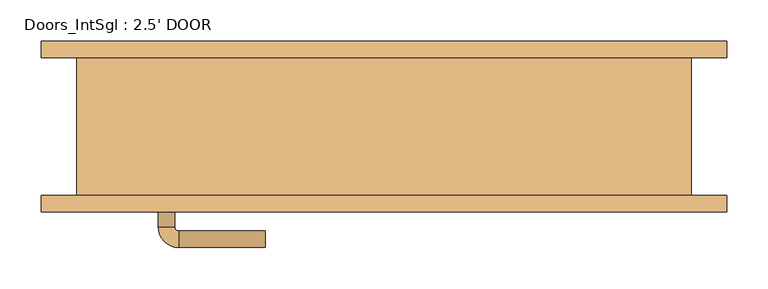
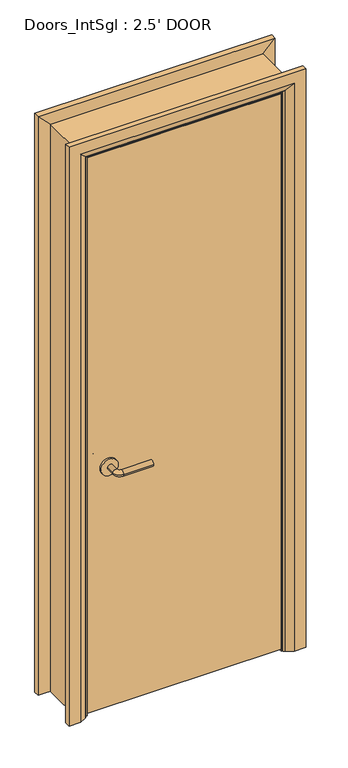
"""IFC4 building model written with IfcOpenShell, lengths in millimetres: door geometry, Doors_IntSgl : 2.5' DOOR."""

from ifc_helpers import new_model, si_unit, point, frame, frame_2d, origin, place, context, project, spatial, polyline, circle_curve, ellipse_curve, trimmed, segment, composite_curve, outline, extrude, faceted_brep, source, transform, mapped, element, save
from ifc_brep_helpers import plane_surface, cylinder_surface, revolved_surface, advanced_brep


def doors_intsgl_2_5_door_57e365e7(model_context):
    return source(origin(), model_context, "Body", "SolidModel", [
        advanced_brep(
        [(-274.0, -37.82, 900.0), (-254.0, -37.82, 900.0), (-274.0, -7.82, 900.0), (-254.0, -7.82, 900.0), (-249.0, -2.82, 900.0), (-249.0, 17.18, 900.0), (-144.0, 17.18, 900.0), (-144.0, -2.82, 900.0)],
        [
            (0, 1, circle_curve(frame((-264.0, -37.82, 900.0), z_axis=(0.0, -1.0, 0.0), x_axis=(1.0, 0.0, 0.0)), 10.0)),
            (1, 0, circle_curve(frame((-264.0, -37.82, 900.0), z_axis=(0.0, -1.0, 0.0), x_axis=(1.0, 0.0, 0.0)), 10.0)),
            (0, 2),
            (2, 3, circle_curve(frame((-264.0, -7.82, 900.0), z_axis=(0.0, -1.0, 0.0), x_axis=(1.0, 0.0, 0.0)), 10.0)),
            (3, 1),
            (3, 2, circle_curve(frame((-264.0, -7.82, 900.0), z_axis=(0.0, -1.0, 0.0), x_axis=(1.0, 0.0, 0.0)), 10.0)),
            (4, 3, circle_curve(frame((-249.0, -7.82, 900.0), z_axis=(0.0, 0.0, 1.0), x_axis=(-1.0, 0.0, 0.0)), 5.0)),
            (2, 5, circle_curve(frame((-249.0, -7.82, 900.0), z_axis=(0.0, 0.0, -1.0), x_axis=(-1.0, 0.0, 0.0)), 25.0)),
            (5, 4, circle_curve(frame((-249.0, 7.18, 900.0), z_axis=(-1.0, 0.0, 0.0), x_axis=(0.0, -1.0, 0.0)), 10.0)),
            (4, 5, circle_curve(frame((-249.0, 7.18, 900.0), z_axis=(-1.0, 0.0, 0.0), x_axis=(0.0, -1.0, 0.0)), 10.0)),
            (6, 7, circle_curve(frame((-144.0, 7.18, 900.0), z_axis=(1.0, 0.0, 0.0), x_axis=(0.0, -1.0, 0.0)), 10.0)),
            (7, 6, circle_curve(frame((-144.0, 7.18, 900.0), z_axis=(1.0, 0.0, 0.0), x_axis=(0.0, -1.0, 0.0)), 10.0)),
            (5, 6),
            (7, 4),
        ],
        [
            plane_surface(frame((-264.0, -37.82, 900.0), z_axis=(0.0, -1.0, 0.0), x_axis=(0.0, 0.0, 1.0))),
            cylinder_surface(frame((-264.0, -37.82, 900.0), z_axis=(0.0, -1.0, 0.0), x_axis=(1.0, 0.0, 0.0)), 10.0),
            revolved_surface(trimmed(ellipse_curve(frame((-264.0, -7.82, 900.0), z_axis=(0.0, -1.0, 0.0), x_axis=(1.0, 0.0, 0.0)), 10.0, 10.0), [point((-274.0, -7.82, 900.0))], [point((-254.0, -7.82, 900.0))], True, "CARTESIAN"), (-249.0, -7.82, 900.0), (0.0, 0.0, -1.0)),
            revolved_surface(trimmed(ellipse_curve(frame((-264.0, -7.82, 900.0), z_axis=(0.0, -1.0, 0.0), x_axis=(1.0, 0.0, 0.0)), 10.0, 10.0), [point((-254.0, -7.82, 900.0))], [point((-274.0, -7.82, 900.0))], True, "CARTESIAN"), (-249.0, -7.82, 900.0), (0.0, 0.0, -1.0)),
            plane_surface(frame((-144.0, 7.18, 900.0), z_axis=(1.0, 0.0, 0.0), x_axis=(0.0, 0.0, 1.0))),
            cylinder_surface(frame((-249.0, 7.18, 900.0), z_axis=(-1.0, 0.0, 0.0), x_axis=(0.0, -1.0, 0.0)), 10.0),
        ],
        [
            (0, [[1, 2]]),
            (1, [[-1, 3, 4, 5]]),
            (1, [[-2, -5, 6, -3]]),
            (2, [[7, -4, 8, 9]]),
            (3, [[-8, -6, -7, 10]]),
            (4, [[11, 12]]),
            (5, [[-9, 13, -12, 14]]),
            (5, [[-10, -14, -11, -13]]),
        ],
    ),
        extrude(outline(composite_curve([segment(trimmed(circle_curve(frame_2d((900.0, -266.5)), 30.0), [point((900.0, -296.5))], [point((900.0, -236.5))], False, "CARTESIAN"), True, "CONTINUOUS"), segment(trimmed(circle_curve(frame_2d((900.0, -266.5)), 30.0), [point((900.0, -236.5))], [point((900.0, -296.5))], False, "CARTESIAN"), True, "CONTINUOUS")], self_intersect=False)), frame((0.0, -45.82, 0.0), z_axis=(0.0, 1.0, 0.0), x_axis=(0.0, 0.0, 1.0)), (0.0, 0.0, 1.0), 8.0),
        advanced_brep(
        [(-274.0, -91.82, 900.0), (-254.0, -91.82, 900.0), (-254.0, -121.82, 900.0), (-274.0, -121.82, 900.0), (-249.0, -126.82, 900.0), (-249.0, -146.82, 900.0), (-144.0, -146.82, 900.0), (-144.0, -126.82, 900.0)],
        [
            (0, 1, circle_curve(frame((-264.0, -91.82, 900.0), z_axis=(0.0, 1.0, 0.0), x_axis=(1.0, 0.0, 0.0)), 10.0)),
            (1, 0, circle_curve(frame((-264.0, -91.82, 900.0), z_axis=(0.0, 1.0, 0.0), x_axis=(1.0, 0.0, 0.0)), 10.0)),
            (1, 2),
            (2, 3, circle_curve(frame((-264.0, -121.82, 900.0), z_axis=(0.0, 1.0, 0.0), x_axis=(1.0, 0.0, 0.0)), 10.0)),
            (3, 0),
            (3, 2, circle_curve(frame((-264.0, -121.82, 900.0), z_axis=(0.0, 1.0, 0.0), x_axis=(1.0, 0.0, 0.0)), 10.0)),
            (4, 5, circle_curve(frame((-249.0, -136.82, 900.0), z_axis=(-1.0, 0.0, 0.0), x_axis=(0.0, 1.0, 0.0)), 10.0)),
            (5, 3, circle_curve(frame((-249.0, -121.82, 900.0), z_axis=(0.0, 0.0, -1.0), x_axis=(-1.0, 0.0, 0.0)), 25.0)),
            (2, 4, circle_curve(frame((-249.0, -121.82, 900.0), z_axis=(0.0, 0.0, 1.0), x_axis=(-1.0, 0.0, 0.0)), 5.0)),
            (5, 4, circle_curve(frame((-249.0, -136.82, 900.0), z_axis=(-1.0, 0.0, 0.0), x_axis=(0.0, 1.0, 0.0)), 10.0)),
            (6, 7, circle_curve(frame((-144.0, -136.82, 900.0), z_axis=(1.0, 0.0, 0.0), x_axis=(0.0, 1.0, 0.0)), 10.0)),
            (7, 6, circle_curve(frame((-144.0, -136.82, 900.0), z_axis=(1.0, 0.0, 0.0), x_axis=(0.0, 1.0, 0.0)), 10.0)),
            (4, 7),
            (6, 5),
        ],
        [
            plane_surface(frame((-264.0, -91.82, 900.0), z_axis=(0.0, 1.0, 0.0), x_axis=(0.0, 0.0, 1.0))),
            cylinder_surface(frame((-264.0, -91.82, 900.0), z_axis=(0.0, 1.0, 0.0), x_axis=(1.0, 0.0, 0.0)), 10.0),
            revolved_surface(trimmed(ellipse_curve(frame((-264.0, -121.82, 900.0), z_axis=(0.0, -1.0, 0.0), x_axis=(1.0, 0.0, 0.0)), 10.0, 10.0), [point((-274.0, -121.82, 900.0))], [point((-254.0, -121.82, 900.0))], True, "CARTESIAN"), (-249.0, -121.82, 900.0), (0.0, 0.0, -1.0)),
            revolved_surface(trimmed(ellipse_curve(frame((-264.0, -121.82, 900.0), z_axis=(0.0, -1.0, 0.0), x_axis=(1.0, 0.0, 0.0)), 10.0, 10.0), [point((-254.0, -121.82, 900.0))], [point((-274.0, -121.82, 900.0))], True, "CARTESIAN"), (-249.0, -121.82, 900.0), (0.0, 0.0, -1.0)),
            plane_surface(frame((-144.0, -136.82, 900.0), z_axis=(1.0, 0.0, 0.0), x_axis=(0.0, 0.0, 1.0))),
            cylinder_surface(frame((-249.0, -136.82, 900.0), z_axis=(-1.0, 0.0, 0.0), x_axis=(0.0, 1.0, 0.0)), 10.0),
        ],
        [
            (0, [[1, 2]]),
            (1, [[3, 4, 5, -2]]),
            (1, [[-5, 6, -3, -1]]),
            (2, [[7, 8, -4, 9]]),
            (3, [[10, -9, -6, -8]]),
            (4, [[11, 12]]),
            (5, [[13, -11, 14, -7]]),
            (5, [[-14, -12, -13, -10]]),
        ],
    ),
        extrude(outline(composite_curve([segment(trimmed(circle_curve(frame_2d((900.0, -266.5)), 30.0), [point((900.0, -296.5))], [point((900.0, -236.5))], False, "CARTESIAN"), True, "CONTINUOUS"), segment(trimmed(circle_curve(frame_2d((900.0, -266.5)), 30.0), [point((900.0, -236.5))], [point((900.0, -296.5))], False, "CARTESIAN"), True, "CONTINUOUS")], self_intersect=False)), frame((0.0, -91.82, 0.0), z_axis=(0.0, 1.0, 0.0), x_axis=(0.0, 0.0, 1.0)), (0.0, 0.0, 1.0), 8.0),
        extrude(outline(polyline([(339.0, -45.82), (339.0, -83.82), (-339.0, -83.82), (-339.0, -45.82), (339.0, -45.82)])), frame((0.0, 0.0, 8.0), z_axis=(0.0, 0.0, 1.0), x_axis=(1.0, 0.0, 0.0)), (0.0, 0.0, 1.0), 2060.0),
        advanced_brep(
        [(416.0, -103.82, 0.0), (376.0, -103.82, 0.0), (350.0, -89.82, 0.0), (346.0, -83.82, 0.0), (416.0, -83.82, 0.0), (416.0, -83.82, 2145.0), (416.0, -103.82, 2145.0), (346.0, -83.82, 2075.0), (-346.0, -83.82, 2075.0), (-346.0, -83.82, 0.0), (-416.0, -83.82, 0.0), (-416.0, -83.82, 2145.0), (350.0, -89.82, 2079.0), (376.0, -103.82, 2105.0), (-416.0, -103.82, 2145.0), (-416.0, -103.82, 0.0), (-376.0, -103.82, 0.0), (-376.0, -103.82, 2105.0), (-350.0, -89.82, 0.0), (-350.0, -89.82, 2079.0)],
        [
            (0, 1),
            (1, 2),
            (2, 3, circle_curve(frame((354.0, -82.82, 0.0), z_axis=(0.0, 0.0, -1.0), x_axis=(1.0, 0.0, 0.0)), 8.0622577)),
            (3, 4),
            (4, 0),
            (4, 5),
            (5, 6),
            (6, 0),
            (3, 7),
            (7, 8),
            (8, 9),
            (9, 10),
            (10, 11),
            (11, 5),
            (2, 12),
            (12, 7, ellipse_curve(frame((354.0, -82.82, 2083.0), z_axis=(0.7071067811865475, 0.0, -0.7071067811865475), x_axis=(-0.7071067811865474, 0.0, -0.7071067811865476)), 11.4017543, 8.0622577)),
            (1, 13),
            (13, 12),
            (6, 14),
            (14, 15),
            (15, 16),
            (16, 17),
            (17, 13),
            (10, 15),
            (14, 11),
            (9, 18, circle_curve(frame((-354.0, -82.82, 0.0), z_axis=(0.0, 0.0, -1.0), x_axis=(-1.0, 0.0, 0.0)), 8.0622577)),
            (18, 16),
            (19, 18),
            (8, 19, ellipse_curve(frame((-354.0, -82.82, 2083.0), z_axis=(-0.7071067811865475, 0.0, -0.7071067811865475), x_axis=(-0.7071067811865474, 0.0, 0.7071067811865476)), 11.4017543, 8.0622577)),
            (19, 17),
            (12, 19),
        ],
        [
            plane_surface(frame((346.0, -83.82, 0.0), z_axis=(0.0, 0.0, -1.0), x_axis=(0.0, 1.0, 0.0))),
            plane_surface(frame((416.0, -103.82, 0.0), z_axis=(1.0, 0.0, 0.0), x_axis=(0.0, 0.0, 1.0))),
            plane_surface(frame((416.0, -83.82, 0.0), z_axis=(0.0, 1.0, 0.0), x_axis=(0.0, 0.0, 1.0))),
            cylinder_surface(frame((354.0, -82.82, 0.0), z_axis=(0.0, 0.0, -1.0), x_axis=(1.0, 0.0, 0.0)), 8.0622577),
            plane_surface(frame((350.0, -89.82, 0.0), z_axis=(-0.4740998230350126, -0.880471099922178, 0.0), x_axis=(0.0, 0.0, 1.0))),
            plane_surface(frame((376.0, -103.82, 0.0), z_axis=(0.0, -1.0, 0.0), x_axis=(0.0, 0.0, 1.0))),
            plane_surface(frame((-416.0, -103.82, 2145.0), z_axis=(-1.0, 0.0, 0.0), x_axis=(0.0, 0.0, -1.0))),
            plane_surface(frame((-346.0, -83.82, 0.0), z_axis=(0.0, 0.0, -1.0), x_axis=(0.0, 1.0, 0.0))),
            cylinder_surface(frame((-354.0, -82.82, 2075.0), z_axis=(0.0, 0.0, 1.0), x_axis=(-1.0, 0.0, 0.0)), 8.0622577),
            plane_surface(frame((-350.0, -89.82, 2079.0), z_axis=(0.47409982303501824, -0.8804710999221749, 0.0), x_axis=(0.0, 0.0, -1.0))),
            plane_surface(frame((416.0, -103.82, 2145.0), z_axis=(0.0, 0.0, 1.0), x_axis=(-1.0, 0.0, 0.0))),
            cylinder_surface(frame((346.0, -82.82, 2083.0), z_axis=(1.0, 0.0, 0.0), x_axis=(0.0, 0.0, 1.0)), 8.0622577),
            plane_surface(frame((350.0, -89.82, 2079.0), z_axis=(0.0, -0.8804710999221764, -0.4740998230350154), x_axis=(-1.0, 0.0, 0.0))),
        ],
        [
            (0, [[1, 2, 3, 4, 5]]),
            (1, [[6, 7, 8, -5]]),
            (2, [[9, 10, 11, 12, 13, 14, -6, -4]]),
            (3, [[15, 16, -9, -3]]),
            (4, [[17, 18, -15, -2]]),
            (5, [[-8, 19, 20, 21, 22, 23, -17, -1]]),
            (6, [[-13, 24, -20, 25]]),
            (7, [[-24, -12, 26, 27, -21]]),
            (8, [[28, -26, -11, 29]]),
            (9, [[-22, -27, -28, 30]]),
            (10, [[-14, -25, -19, -7]]),
            (11, [[31, -29, -10, -16]]),
            (12, [[-23, -30, -31, -18]]),
        ],
    ),
        extrude(outline(polyline([(0.0, -322.0), (2051.0, -322.0), (2051.0, 322.0), (0.0, 322.0), (0.0, 341.0), (2070.0, 341.0), (2070.0, -341.0), (0.0, -341.0), (0.0, -322.0)])), frame((0.0, -43.82, 0.0), z_axis=(0.0, 1.0, 0.0), x_axis=(0.0, 0.0, 1.0)), (0.0, 0.0, 1.0), 32.0),
        advanced_brep(
        [(-416.0, 103.82, 0.0), (-376.0, 103.82, 0.0), (-350.0, 89.82, 0.0), (-346.0, 83.82, 0.0), (-416.0, 83.82, 0.0), (-416.0, 83.82, 2145.0), (-416.0, 103.82, 2145.0), (-346.0, 83.82, 2075.0), (-350.0, 89.82, 2079.0), (-376.0, 103.82, 2105.0), (416.0, 103.82, 0.0), (416.0, 83.82, 0.0), (346.0, 83.82, 0.0), (350.0, 89.82, 0.0), (376.0, 103.82, 0.0), (416.0, 103.82, 2145.0), (376.0, 103.82, 2105.0), (350.0, 89.82, 2079.0), (346.0, 83.82, 2075.0), (416.0, 83.82, 2145.0)],
        [
            (0, 1),
            (1, 2),
            (2, 3, circle_curve(frame((-354.0, 82.82, 0.0), z_axis=(0.0, 0.0, -1.0), x_axis=(-1.0, 0.0, 0.0)), 8.0622577)),
            (3, 4),
            (4, 0),
            (4, 5),
            (5, 6),
            (6, 0),
            (3, 7),
            (7, 5),
            (2, 8),
            (8, 7, ellipse_curve(frame((-354.0, 82.82, 2083.0), z_axis=(-0.7071067811865475, 0.0, -0.7071067811865475), x_axis=(0.7071067811865474, 0.0, -0.7071067811865476)), 11.4017543, 8.0622577)),
            (1, 9),
            (9, 8),
            (6, 9),
            (10, 11),
            (11, 12),
            (12, 13, circle_curve(frame((354.0, 82.82, 0.0), z_axis=(0.0, 0.0, -1.0), x_axis=(1.0, 0.0, 0.0)), 8.0622577)),
            (13, 14),
            (14, 10),
            (15, 10),
            (14, 16),
            (16, 15),
            (13, 17),
            (17, 16),
            (12, 18),
            (18, 17, ellipse_curve(frame((354.0, 82.82, 2083.0), z_axis=(0.7071067811865475, 0.0, -0.7071067811865475), x_axis=(0.7071067811865474, 0.0, 0.7071067811865476)), 11.4017543, 8.0622577)),
            (11, 19),
            (19, 18),
            (15, 19),
            (5, 19),
            (15, 6),
            (7, 18),
            (8, 17),
            (9, 16),
        ],
        [
            plane_surface(frame((-346.0, 156.6210989, 0.0), z_axis=(0.0, 0.0, -1.0), x_axis=(1.0, 0.0, 0.0))),
            plane_surface(frame((-416.0, 103.82, 0.0), z_axis=(-1.0, 0.0, 0.0), x_axis=(0.0, 0.0, 1.0))),
            plane_surface(frame((-416.0, 83.82, 0.0), z_axis=(0.0, -1.0, 0.0), x_axis=(0.0, 0.0, 1.0))),
            cylinder_surface(frame((-354.0, 82.82, 0.0), z_axis=(0.0, 0.0, -1.0), x_axis=(-1.0, 0.0, 0.0)), 8.0622577),
            plane_surface(frame((-350.0, 89.82, 0.0), z_axis=(0.4740998230350183, 0.8804710999221749, 0.0), x_axis=(0.0, 0.0, 1.0))),
            plane_surface(frame((-376.0, 103.82, 0.0), z_axis=(0.0, 1.0, 0.0), x_axis=(0.0, 0.0, 1.0))),
            plane_surface(frame((346.0, 156.6210989, 0.0), z_axis=(0.0, 0.0, -1.0), x_axis=(-1.0, 0.0, 0.0))),
            plane_surface(frame((376.0, 103.82, 2105.0), z_axis=(0.0, 1.0, 0.0), x_axis=(0.0, 0.0, -1.0))),
            plane_surface(frame((350.0, 89.82, 2079.0), z_axis=(-0.4740998230350183, 0.8804710999221749, 0.0), x_axis=(0.0, 0.0, -1.0))),
            cylinder_surface(frame((354.0, 82.82, 2075.0), z_axis=(0.0, 0.0, 1.0), x_axis=(1.0, 0.0, 0.0)), 8.0622577),
            plane_surface(frame((416.0, 83.82, 2145.0), z_axis=(0.0, -1.0, 0.0), x_axis=(0.0, 0.0, -1.0))),
            plane_surface(frame((416.0, 103.82, 2145.0), z_axis=(1.0, 0.0, 0.0), x_axis=(0.0, 0.0, -1.0))),
            plane_surface(frame((-416.0, 103.82, 2145.0), z_axis=(0.0, 0.0, 1.0), x_axis=(1.0, 0.0, 0.0))),
            plane_surface(frame((-416.0, 83.82, 2145.0), z_axis=(0.0, -1.0, 0.0), x_axis=(1.0, 0.0, 0.0))),
            cylinder_surface(frame((-346.0, 82.82, 2083.0), z_axis=(-1.0, 0.0, 0.0), x_axis=(0.0, 0.0, 1.0)), 8.0622577),
            plane_surface(frame((-350.0, 89.82, 2079.0), z_axis=(0.0, 0.8804710999221749, -0.4740998230350183), x_axis=(1.0, 0.0, 0.0))),
            plane_surface(frame((-376.0, 103.82, 2105.0), z_axis=(0.0, 1.0, 0.0), x_axis=(1.0, 0.0, 0.0))),
        ],
        [
            (0, [[1, 2, 3, 4, 5]]),
            (1, [[6, 7, 8, -5]]),
            (2, [[9, 10, -6, -4]]),
            (3, [[11, 12, -9, -3]]),
            (4, [[13, 14, -11, -2]]),
            (5, [[-8, 15, -13, -1]]),
            (6, [[16, 17, 18, 19, 20]]),
            (7, [[21, -20, 22, 23]]),
            (8, [[-22, -19, 24, 25]]),
            (9, [[-24, -18, 26, 27]]),
            (10, [[-26, -17, 28, 29]]),
            (11, [[-28, -16, -21, 30]]),
            (12, [[31, -30, 32, -7]]),
            (13, [[33, -29, -31, -10]]),
            (14, [[34, -27, -33, -12]]),
            (15, [[35, -25, -34, -14]]),
            (16, [[-32, -23, -35, -15]]),
        ],
    ),
        faceted_brep([(-341.0, -83.82, 0.0), (-373.0, -83.82, 0.0), (-373.0, 83.82, 0.0), (-341.0, 83.82, 0.0), (-341.0, 83.82, 2070.0), (-341.0, -83.82, 2070.0), (-373.0, 83.82, 2102.0), (-373.0, -83.82, 2102.0), (341.0, -83.82, 0.0), (341.0, 83.82, 0.0), (373.0, 83.82, 0.0), (373.0, -83.82, 0.0), (341.0, -83.82, 2070.0), (373.0, -83.82, 2102.0), (373.0, 83.82, 2102.0), (341.0, 83.82, 2070.0)], [[[0, 1, 2, 3]], [[3, 4, 5, 0]], [[2, 6, 4, 3]], [[1, 7, 6, 2]], [[0, 5, 7, 1]], [[8, 9, 10, 11]], [[12, 8, 11, 13]], [[13, 11, 10, 14]], [[14, 10, 9, 15]], [[15, 9, 8, 12]], [[4, 15, 12, 5]], [[6, 14, 15, 4]], [[7, 13, 14, 6]], [[5, 12, 13, 7]]]),
    ])


if __name__ == "__main__":
    model = new_model("IFC4")
    model_context = context("Model", 3, world=origin())
    ifc_project = project(units=[si_unit("LENGTHUNIT", "METRE", prefix="MILLI")], contexts=[model_context])
    site = spatial("IfcSite", under=ifc_project)
    building = spatial("IfcBuilding", under=site)
    placement = place(None, origin())
    doors_intsgl_2_5_door_shape = doors_intsgl_2_5_door_57e365e7(model_context)
    element("IfcDoor", 1, ObjectType="Doors_IntSgl : 2.5' DOOR", at=placement, inside=building, context=model_context, shape_type="MappedRepresentation", body=[
        mapped(doors_intsgl_2_5_door_shape, transform((0.0, 0.0, 0.0), x_axis=(1.0, 0.0, 0.0), y_axis=(0.0, 1.0, 0.0), z_axis=(0.0, 0.0, 1.0))),
    ])
    save(model, "model.ifc")

# Revit data of these elements
# Type "Doors_IntSgl : 2.5' DOOR"
#   Type Mark = "47"
#   Type Comments = "Internal Single"
#   Operation = "SingleSwingRight"
#   Manufacturer = "Revit"
#   Keynote = "L20"
#   Description = "Internal Single Door"
#   Analytic Construction = "Metal"
#   UnderCut = 0.026247 ft
#   Tolerance = 0.006562 ft
#   Thickness = 0.124672 ft
#   Thermal Resistance (R) = 0.270117 (m²·K)/W
#   Structural Tolerance = 0.026247 ft
#   StopDepth = 0.104987 ft
#   Stop Thickness = 0.062336 ft
#   Rough Width = 2.5 ft
#   Rough Height = 6.922572 ft
#   Height to Top Lock Rail = 3.28084 ft
#   Heat Transfer Coefficient (U) = 3.7021 W/(m²·K)
#   Handle Z Distance = 2.952756 ft
#   Handle X Distance = 0.246063 ft
#   Frame Thickness = 0.104987 ft
#   Door Panel Width = 2.224409 ft
#   Door Panel Thickness = 0.124672 ft
#   Door Panel Offset = 0.0 ft
#   Height = 6.922572 ft
#   Width = 2.5 ft
#   Door Panel Height = 6.75853 ft
#   Architrave Setback = 0.016404 ft
#   Vis - Ironmongery = yes
#   Material Ironmongery = Door - Handle
#   Material Frame = Door - Frame/Mullion (1)
#   Material Door = Door - Panel
#   Material Architrave = Door - Architrave
#   Visual Light Transmittance = 0
#   Solar Heat Gain Coefficient = 0
#   Function = (empty or 0)
#   Wall Closure = (empty or 0)
# Element 1 (IfcDoor, "Doors_IntSgl : 2.5' DOOR")
#   Materials on its faces: "Door - Architrave", "Door - Handle", "Door - Frame/Mullion (1)", "Door - Panel"
# Materials
#   "Door - Handle": colour RGB 0 0 0, transparency 0, Keynote = "P21", Cost = 0
#   "Door - Frame/Mullion (1)": class "Wood", colour RGB 212 179 113, transparency 0, Keynote = "L20", Cost = 0
#   "Door - Panel": class "Wood", colour RGB 210 159 95, transparency 0, Keynote = "L20", Cost = 0
#   "Door - Architrave": class "Wood", colour RGB 154 90 5, transparency 0, Keynote = "P20", Cost = 0
